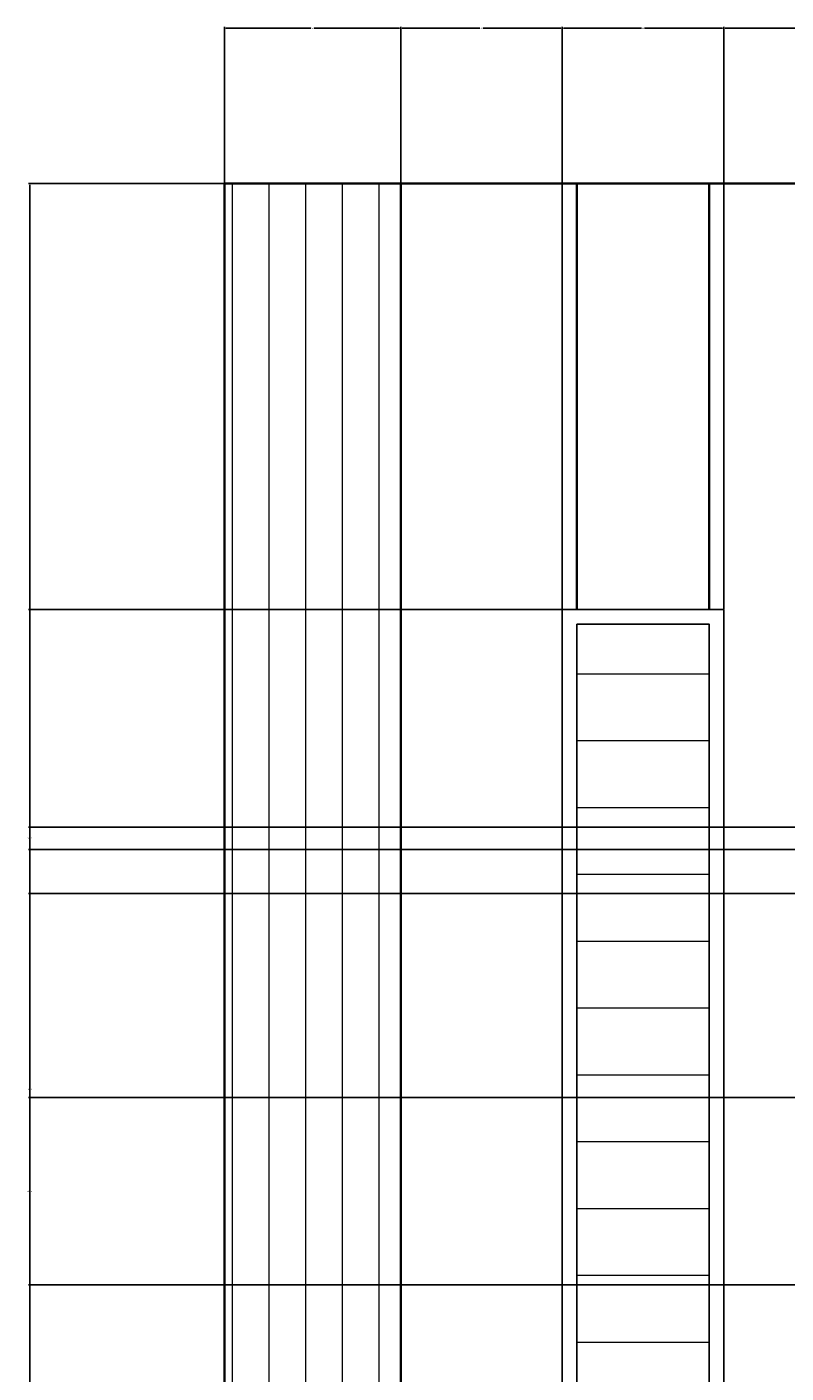
# Model space of a CAD drawing. Units: inches. Extents: x -3 to 302, y -138 to 325.
# Tile 4 of 5: x -3 to 100, y 141 to 325. Entities that reach past the tile are written whole.
import ezdxf

# ---------------------------------------------------------------- set-up
doc = ezdxf.new("R2010")
doc.units = ezdxf.units.IN
doc.header["$MEASUREMENT"] = 0
for name, color, linetype, lineweight in [('A-ANNO-DIMS', 2, 'Continuous', 18), ('A-ELEV', 7, 'Continuous', 35), ('A-ELEV-PATT', 8, 'Continuous', 13), ('A-GLAZ', 3, 'Continuous', 25)]:
    doc.layers.add(name, color=color, linetype=linetype, lineweight=lineweight)
doc.styles.get("Standard").update_dxf_attribs({"font": 'arial.ttf'})
doc.dimstyles.get("Standard").update_dxf_attribs({"dimtxt": 0.18, "dimasz": 0.18, "dimexe": 0.18, "dimexo": 0.0625, "dimgap": 0.09, "dimtad": 0, "dimtih": 1, "dimtoh": 1, "dimdec": 4, "dimzin": 0, "dimdsep": 46, "dimtxsty": 'Standard', "dimcen": 0.09, "dimadec": 0, "dimazin": 0, "dimtfac": 1, "dimtdec": 4, "dimtofl": 0, "dimtmove": 0, "dimatfit": 3, "dimfxl": 1, "dimtolj": 1, "dimtzin": 0, "dimarcsym": 0})

# ---------------------------------------------------------------- blocks, each defined once
blk = doc.blocks.new('*D18')
at = {"layer": 'A-ANNO-DIMS', "color": 0, "lineweight": -2, "transparency": 16777216}
for p, q in [((23.86, 303.37), (-2.8, 303.37)), ((-2.62, 303.19), (-2.62, 93.56)), ((-2.62, -116.45), (-2.62, 93.19)), ((23.86, -116.63), (-2.8, -116.63))]:
    blk.add_line(p, q, dxfattribs=at)
at = {"layer": 'A-ANNO-DIMS', "color": 0, "transparency": 16777216}
for points in [[(-2.65, 303.19), (-2.59, 303.19), (-2.62, 303.37)], [(-2.65, -116.45), (-2.59, -116.45), (-2.62, -116.63)]]:
    blk.add_solid(points, dxfattribs=at)
at = {"layer": 'Defpoints', "color": 0, "transparency": 16777216}
for p in [(-2.62, 303.37), (23.92, 303.37), (23.92, -116.63)]:
    blk.add_point(p, dxfattribs=at)
at = {"layer": 'A-ANNO-DIMS', "color": 0, "transparency": 16777216, "insert": (-2.62, 93.37), "char_height": 0.18, "attachment_point": 5}
blk.add_mtext('\\A1;420', dxfattribs=at)
blk = doc.blocks.new('*D24')
at = {"layer": 'A-ANNO-DIMS', "color": 0, "lineweight": -2, "transparency": 16777216}
for p, q in [((23.92, 303.44), (23.92, 324.7)), ((24.1, 324.52), (35.7, 324.52)), ((47.74, 324.52), (36.14, 324.52)), ((47.92, 303.44), (47.92, 324.7))]:
    blk.add_line(p, q, dxfattribs=at)
at = {"layer": 'A-ANNO-DIMS', "color": 0, "transparency": 16777216}
for points in [[(24.1, 324.55), (24.1, 324.49), (23.92, 324.52)], [(47.74, 324.55), (47.74, 324.49), (47.92, 324.52)]]:
    blk.add_solid(points, dxfattribs=at)
at = {"layer": 'Defpoints', "color": 0, "transparency": 16777216}
for p in [(47.92, 324.52), (23.92, 303.37), (47.92, 303.37)]:
    blk.add_point(p, dxfattribs=at)
at = {"layer": 'A-ANNO-DIMS', "color": 0, "transparency": 16777216, "insert": (35.92, 324.52), "char_height": 0.18, "attachment_point": 5}
blk.add_mtext('\\A1;24', dxfattribs=at)
blk = doc.blocks.new('*D25')
at = {"layer": 'A-ANNO-DIMS', "color": 0, "lineweight": -2, "transparency": 16777216}
for p, q in [((47.92, 303.44), (47.92, 324.7)), ((48.1, 324.52), (58.7, 324.52)), ((69.74, 324.52), (59.14, 324.52)), ((69.92, 245.44), (69.92, 324.7))]:
    blk.add_line(p, q, dxfattribs=at)
at = {"layer": 'A-ANNO-DIMS', "color": 0, "transparency": 16777216}
for points in [[(48.1, 324.55), (48.1, 324.49), (47.92, 324.52)], [(69.74, 324.55), (69.74, 324.49), (69.92, 324.52)]]:
    blk.add_solid(points, dxfattribs=at)
at = {"layer": 'Defpoints', "color": 0, "transparency": 16777216}
for p in [(69.92, 324.52), (47.92, 303.37), (69.92, 245.37)]:
    blk.add_point(p, dxfattribs=at)
at = {"layer": 'A-ANNO-DIMS', "color": 0, "transparency": 16777216, "insert": (58.92, 324.52), "char_height": 0.18, "attachment_point": 5}
blk.add_mtext('\\A1;22', dxfattribs=at)
blk = doc.blocks.new('*D26')
at = {"layer": 'A-ANNO-DIMS', "color": 0, "lineweight": -2, "transparency": 16777216}
for p, q in [((69.92, 245.44), (69.92, 324.7)), ((70.1, 324.52), (80.7, 324.52)), ((91.74, 324.52), (81.14, 324.52)), ((91.92, 245.44), (91.92, 324.7))]:
    blk.add_line(p, q, dxfattribs=at)
at = {"layer": 'A-ANNO-DIMS', "color": 0, "transparency": 16777216}
for points in [[(70.1, 324.55), (70.1, 324.49), (69.92, 324.52)], [(91.74, 324.55), (91.74, 324.49), (91.92, 324.52)]]:
    blk.add_solid(points, dxfattribs=at)
at = {"layer": 'Defpoints', "color": 0, "transparency": 16777216}
for p in [(91.92, 324.52), (69.92, 245.37), (91.92, 245.37)]:
    blk.add_point(p, dxfattribs=at)
at = {"layer": 'A-ANNO-DIMS', "color": 0, "transparency": 16777216, "insert": (80.92, 324.52), "char_height": 0.18, "attachment_point": 5}
blk.add_mtext('\\A1;22', dxfattribs=at)
blk = doc.blocks.new('*D27')
at = {"layer": 'A-ANNO-DIMS', "color": 0, "lineweight": -2, "transparency": 16777216}
for p, q in [((91.92, 245.44), (91.92, 324.7)), ((92.1, 324.52), (102.7, 324.52)), ((113.74, 324.52), (103.14, 324.52)), ((113.92, 303.44), (113.92, 324.7))]:
    blk.add_line(p, q, dxfattribs=at)
at = {"layer": 'A-ANNO-DIMS', "color": 0, "transparency": 16777216}
for points in [[(92.1, 324.55), (92.1, 324.49), (91.92, 324.52)], [(113.74, 324.55), (113.74, 324.49), (113.92, 324.52)]]:
    blk.add_solid(points, dxfattribs=at)
at = {"layer": 'Defpoints', "color": 0, "transparency": 16777216}
for p in [(113.92, 324.52), (113.92, 303.37), (91.92, 245.37)]:
    blk.add_point(p, dxfattribs=at)
at = {"layer": 'A-ANNO-DIMS', "color": 0, "transparency": 16777216, "insert": (102.92, 324.52), "char_height": 0.18, "attachment_point": 5}
blk.add_mtext('\\A1;22', dxfattribs=at)
blk = doc.blocks.new('*D37')
at = {"layer": 'A-ANNO-DIMS', "color": 0, "lineweight": -2, "transparency": 16777216}
for p, q in [((69.86, 245.37), (-2.8, 245.37)), ((-2.62, 245.19), (-2.62, 105.73)), ((-2.62, -34.09), (-2.62, 105.37)), ((69.86, -34.27), (-2.8, -34.27))]:
    blk.add_line(p, q, dxfattribs=at)
at = {"layer": 'A-ANNO-DIMS', "color": 0, "transparency": 16777216}
for points in [[(-2.65, 245.19), (-2.59, 245.19), (-2.62, 245.37)], [(-2.65, -34.09), (-2.59, -34.09), (-2.62, -34.27)]]:
    blk.add_solid(points, dxfattribs=at)
at = {"layer": 'Defpoints', "color": 0, "transparency": 16777216}
for p in [(-2.62, 245.37), (69.92, 245.37), (69.92, -34.27)]:
    blk.add_point(p, dxfattribs=at)
at = {"layer": 'A-ANNO-DIMS', "color": 0, "transparency": 16777216, "insert": (-2.62, 105.55), "char_height": 0.18, "attachment_point": 5}
blk.add_mtext('\\A1;279.65', dxfattribs=at)
blk = doc.blocks.new('*D38')
at = {"layer": 'A-ANNO-DIMS', "color": 0, "lineweight": -2, "transparency": 16777216}
for p, q in [((71.86, 303.37), (-2.8, 303.37)), ((-2.62, 303.19), (-2.62, 274.56)), ((-2.62, 245.55), (-2.62, 274.19)), ((69.86, 245.37), (-2.8, 245.37))]:
    blk.add_line(p, q, dxfattribs=at)
at = {"layer": 'A-ANNO-DIMS', "color": 0, "transparency": 16777216}
for points in [[(-2.65, 303.19), (-2.59, 303.19), (-2.62, 303.37)], [(-2.65, 245.55), (-2.59, 245.55), (-2.62, 245.37)]]:
    blk.add_solid(points, dxfattribs=at)
at = {"layer": 'Defpoints', "color": 0, "transparency": 16777216}
for p in [(-2.62, 303.37), (71.92, 303.37), (69.92, 245.37)]:
    blk.add_point(p, dxfattribs=at)
at = {"layer": 'A-ANNO-DIMS', "color": 0, "transparency": 16777216, "insert": (-2.62, 274.37), "char_height": 0.18, "attachment_point": 5}
blk.add_mtext('\\A1;58', dxfattribs=at)
blk = doc.blocks.new('*D60')
at = {"layer": 'A-ANNO-DIMS', "color": 0, "lineweight": -2, "transparency": 16777216}
for p, q in [((146.02, 206.67), (-2.8, 206.67)), ((-2.62, 206.49), (-2.62, 180.21)), ((-2.62, 153.55), (-2.62, 179.84)), ((139.02, 153.37), (-2.8, 153.37))]:
    blk.add_line(p, q, dxfattribs=at)
at = {"layer": 'A-ANNO-DIMS', "color": 0, "transparency": 16777216}
for points in [[(-2.65, 206.49), (-2.59, 206.49), (-2.62, 206.67)], [(-2.65, 153.55), (-2.59, 153.55), (-2.62, 153.37)]]:
    blk.add_solid(points, dxfattribs=at)
at = {"layer": 'Defpoints', "color": 0, "transparency": 16777216}
for p in [(-2.62, 206.67), (146.09, 206.67), (139.09, 153.37)]:
    blk.add_point(p, dxfattribs=at)
at = {"layer": 'A-ANNO-DIMS', "color": 0, "transparency": 16777216, "insert": (-2.62, 180.02), "char_height": 0.18, "attachment_point": 5}
blk.add_mtext('\\A1;53.3', dxfattribs=at)
blk = doc.blocks.new('*D61')
at = {"layer": 'A-ANNO-DIMS', "color": 0, "lineweight": -2, "transparency": 16777216}
for p, q in [((142.02, 212.67), (-2.8, 212.67)), ((-2.62, 212.49), (-2.62, 209.86)), ((-2.62, 206.85), (-2.62, 209.49)), ((146.02, 206.67), (-2.8, 206.67))]:
    blk.add_line(p, q, dxfattribs=at)
at = {"layer": 'A-ANNO-DIMS', "color": 0, "transparency": 16777216}
for points in [[(-2.65, 212.49), (-2.59, 212.49), (-2.62, 212.67)], [(-2.65, 206.85), (-2.59, 206.85), (-2.62, 206.67)]]:
    blk.add_solid(points, dxfattribs=at)
at = {"layer": 'Defpoints', "color": 0, "transparency": 16777216}
for p in [(-2.62, 212.67), (142.09, 212.67), (146.09, 206.67)]:
    blk.add_point(p, dxfattribs=at)
at = {"layer": 'A-ANNO-DIMS', "color": 0, "transparency": 16777216, "insert": (-2.62, 209.67), "char_height": 0.18, "attachment_point": 5}
blk.add_mtext('\\A1;6', dxfattribs=at)
blk = doc.blocks.new('*D62')
at = {"layer": 'A-ANNO-DIMS', "color": 0, "lineweight": -2, "transparency": 16777216}
for p, q in [((139.02, 215.7), (-2.8, 215.7)), ((-2.62, 215.52), (-2.62, 214.37)), ((142.02, 212.67), (-2.8, 212.67)), ((-2.62, 212.85), (-2.62, 214))]:
    blk.add_line(p, q, dxfattribs=at)
at = {"layer": 'A-ANNO-DIMS', "color": 0, "transparency": 16777216}
for points in [[(-2.65, 215.52), (-2.59, 215.52), (-2.62, 215.7)], [(-2.65, 212.85), (-2.59, 212.85), (-2.62, 212.67)]]:
    blk.add_solid(points, dxfattribs=at)
at = {"layer": 'Defpoints', "color": 0, "transparency": 16777216}
for p in [(-2.62, 215.7), (139.09, 215.7), (142.09, 212.67)]:
    blk.add_point(p, dxfattribs=at)
at = {"layer": 'A-ANNO-DIMS', "color": 0, "transparency": 16777216, "insert": (-2.62, 214.19), "char_height": 0.18, "attachment_point": 5}
blk.add_mtext('\\A1;3.023', dxfattribs=at)
blk = doc.blocks.new('*D63')
at = {"layer": 'A-ANNO-DIMS', "color": 0, "lineweight": -2, "transparency": 16777216}
for p, q in [((169.52, 178.91), (-2.8, 178.91)), ((-2.62, 178.73), (-2.62, 166.33)), ((-2.62, 153.55), (-2.62, 165.96)), ((168.02, 153.37), (-2.8, 153.37))]:
    blk.add_line(p, q, dxfattribs=at)
at = {"layer": 'A-ANNO-DIMS', "color": 0, "transparency": 16777216}
for points in [[(-2.65, 178.73), (-2.59, 178.73), (-2.62, 178.91)], [(-2.65, 153.55), (-2.59, 153.55), (-2.62, 153.37)]]:
    blk.add_solid(points, dxfattribs=at)
at = {"layer": 'Defpoints', "color": 0, "transparency": 16777216}
for p in [(-2.62, 178.91), (169.58, 178.91), (168.09, 153.37)]:
    blk.add_point(p, dxfattribs=at)
at = {"layer": 'A-ANNO-DIMS', "color": 0, "transparency": 16777216, "insert": (-2.62, 166.14), "char_height": 0.18, "attachment_point": 5}
blk.add_mtext('\\A1;25.54', dxfattribs=at)

msp = doc.modelspace()

# ---------------------------------------------------------------- hatches: boundary and pattern name
at = {"layer": 'A-ELEV-PATT'}
h = msp.add_hatch(dxfattribs=at)
h.set_pattern_fill('_USER', color=256, scale=5, angle=90, pattern_type=0)
h.set_pattern_definition([(90, (0, 0), (-5, 3e-16), [])])
h.paths.add_polyline_path([(47.922, 303.3747), (23.922, 303.3747), (23.922, 123.3747), (23.922, 3.3747), (23.922, -49.0923), (47.922, -49.0923)])
h = msp.add_hatch(dxfattribs=at)
h.set_pattern_fill('_USER', color=256, scale=9.1, pattern_type=0)
h.set_pattern_definition([(0, (0, 0), (0, 9.1), [])])
h.paths.add_polyline_path([(89.922, 243.3747), (71.922, 243.3747), (71.922, -32.2717), (89.922, -32.2717)])

# ---------------------------------------------------------------- linework, layer by layer
at = {"layer": 'A-ELEV'}
for p, q in [((23.922, 123.3747), (23.922, 303.3747)), ((23.922, 303.3747), (113.922, 303.3747)), ((47.922, 303.3747), (47.922, -49.0923)), ((71.922, 303.3747), (71.922, 245.3747)), ((89.922, 245.3747), (89.922, 303.3747))]:
    msp.add_line(p, q, dxfattribs=at)
at = {"layer": 'A-GLAZ'}
for points in [[(69.922, 245.3747), (69.922, -34.2717), (91.922, -34.2717), (91.922, 245.3747)], [(71.922, 243.3747), (71.922, -32.2717), (89.922, -32.2717), (89.922, 243.3747)]]:
    msp.add_lwpolyline(points, close=True, dxfattribs=at)

# ---------------------------------------------------------------- dimensions: what is measured, and where the dimension line sits
at = {"layer": 'A-ANNO-DIMS'}
for base, p1, p2, picture, middle in [((47.922, 324.5247), (23.922, 303.3747), (47.922, 303.3747), '*D24', (35.922, 324.5247)), ((69.922, 324.5247), (47.922, 303.3747), (69.922, 245.3747), '*D25', (58.922, 324.5247)), ((91.922, 324.5247), (69.922, 245.3747), (91.922, 245.3747), '*D26', (80.922, 324.5247)), ((113.922, 324.5247), (91.922, 245.3747), (113.922, 303.3747), '*D27', (102.922, 324.5247))]:
    dim = msp.add_linear_dim(base=base, p1=p1, p2=p2, dimstyle='Standard', override={"dimdec": 0, "dimlfac": 1, "dimrnd": 0, "dimzin": 0, "dimdsep": 46, "dimlunit": 2}, dxfattribs=at)
    dim.commit()
    dim.dimension.update_dxf_attribs({"geometry": picture, "text_midpoint": middle})
for base, p1, p2, override, picture, middle in [((-2.6197, 303.3747), (23.922, -116.6253), (23.922, 303.3747), {"dimdec": 0, "dimlfac": 1, "dimrnd": 0, "dimzin": 0, "dimdsep": 46, "dimlunit": 2}, '*D18', (-2.6197, 93.3747)), ((-2.6197, 303.3747), (69.922, 245.3747), (71.922, 303.3747), {"dimdec": 0, "dimlfac": 1, "dimrnd": 0, "dimzin": 0, "dimdsep": 46, "dimlunit": 2}, '*D38', (-2.6197, 274.3747)), ((-2.6197, 245.3747), (69.922, -34.2717), (69.922, 245.3747), {"dimdec": 2, "dimlfac": 1, "dimrnd": 0, "dimzin": 0, "dimdsep": 46, "dimlunit": 2}, '*D37', (-2.6197, 105.5515)), ((-2.6197, 215.6966), (142.0861, 212.6736), (139.0861, 215.6966), {"dimdec": 3, "dimlfac": 1, "dimrnd": 0, "dimzin": 0, "dimdsep": 46, "dimlunit": 2}, '*D62', (-2.6197, 214.1851)), ((-2.6197, 212.6736), (146.0861, 206.6736), (142.0861, 212.6736), {"dimdec": 0, "dimlfac": 1, "dimrnd": 0, "dimzin": 0, "dimdsep": 46, "dimlunit": 2}, '*D61', (-2.6197, 209.6736)), ((-2.6197, 206.6736), (139.0861, 153.3747), (146.0861, 206.6736), {"dimdec": 1, "dimlfac": 1, "dimrnd": 0, "dimzin": 0, "dimdsep": 46, "dimlunit": 2}, '*D60', (-2.6197, 180.0242)), ((-2.6197, 178.9138), (168.0861, 153.3747), (169.5811, 178.9138), {"dimdec": 2, "dimlfac": 1, "dimrnd": 0, "dimzin": 0, "dimdsep": 46, "dimlunit": 2}, '*D63', (-2.6197, 166.1442))]:
    dim = msp.add_linear_dim(base=base, p1=p1, p2=p2, angle=90, dimstyle='Standard', override=override, dxfattribs=at)
    dim.commit()
    dim.dimension.update_dxf_attribs({"geometry": picture, "text_midpoint": middle})

doc.saveas('drawing.dxf')
